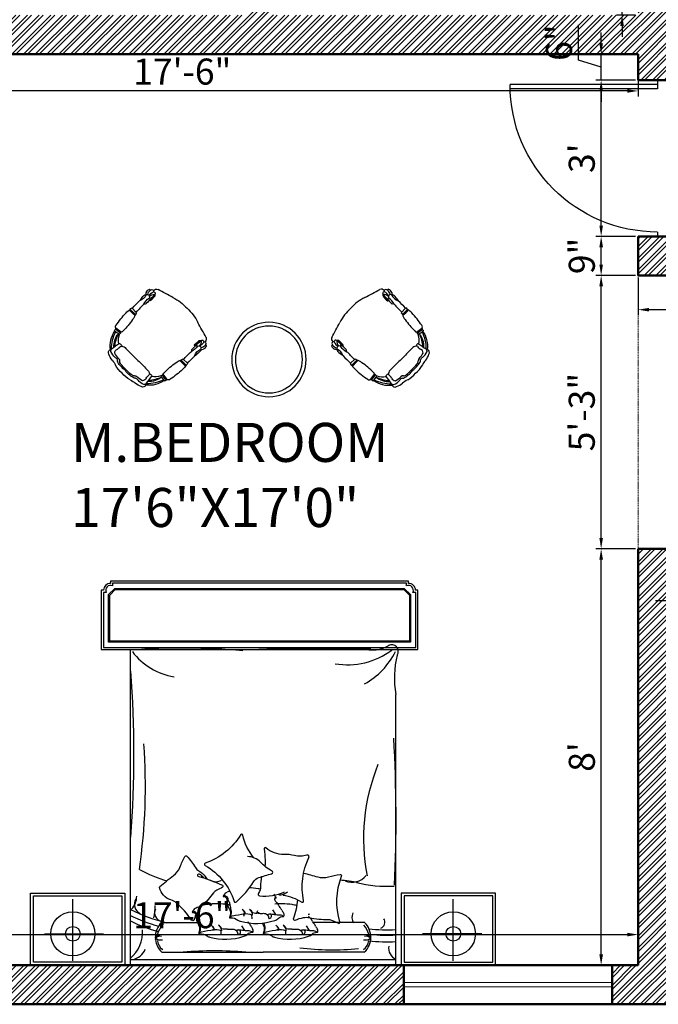
# Model space of a CAD drawing. Units: inches. Extents: x 3590 to 5167, y 65 to 1917.
# Tile 8 of 100: x 4497 to 4644, y 109 to 336. Entities that reach past the tile are written whole.
import ezdxf

# ---------------------------------------------------------------- set-up
doc = ezdxf.new("R2010")
doc.units = ezdxf.units.IN
doc.linetypes.add('DASHED', pattern=[0.75, 0.5, -0.25])
for name, color, linetype, lineweight in [('A-ANNO-DIMS', 2, 'Continuous', 18), ('A-AREA-IDEN', 7, 'Continuous', 18), ('A-DOOR', 3, 'Continuous', 25), ('A-FURN', 21, 'Continuous', 18), ('A-GLAZ', 4, 'Continuous', 18), ('A-WALL', 7, 'Continuous', 50), ('A-WALL-PATT', 251, 'Continuous', 13), ('S-BEAM-OVHD', 7, 'DASHED', 18)]:
    doc.layers.add(name, color=color, linetype=linetype, lineweight=lineweight)
for name, color, linetype in [('FUR', 42, 'Continuous'), ('furn', 7, 'Continuous'), ('HA-FUR', 8, 'Continuous'), ('HA-P', 8, 'Continuous'), ('SAN', 5, 'Continuous'), ('wood', 26, 'Continuous')]:
    doc.layers.add(name, color=color, linetype=linetype)
doc.styles.get("Standard").update_dxf_attribs({"font": 'arial.ttf'})
doc.dimstyles.new('ISO-25', dxfattribs={"dimtxt": 9, "dimasz": 2.5, "dimexe": 1.25, "dimexo": 0.625, "dimtad": 1, "dimdec": 1, "dimlunit": 3, "dimtxsty": 'Standard', "dimcen": 2.5, "dimadec": 0, "dimazin": 0, "dimtfac": 1, "dimtdec": 1, "dimtmove": 0, "dimatfit": 3, "dimfxl": 1, "dimarcsym": 0})

# ---------------------------------------------------------------- blocks, each defined once
blk = doc.blocks.new('D1')
for p, q in [((1, 0), (1, 34)), ((2, 0), (2, 33.99)), ((0, 0), (2, 0)), ((35, 0), (36, 0))]:
    blk.add_line(p, q)
at = {"ltscale": 0.5}
blk.add_arc((1, 0), 34, 0, 90, dxfattribs=at)
blk = doc.blocks.new('*D262')
at = {"layer": 'A-ANNO-DIMS', "color": 0, "lineweight": -2, "transparency": 16777216}
for p, q in [((4635.58, 345.56), (4635.58, 356.24)), ((4638.65, 343.06), (4634.33, 343.06)), ((4635.58, 337.06), (4635.58, 343.06)), ((4638.65, 337.06), (4634.33, 337.06)), ((4635.58, 334.56), (4635.58, 332.06))]:
    blk.add_line(p, q, dxfattribs=at)
at = {"layer": 'A-ANNO-DIMS', "color": 0, "transparency": 16777216}
for points in [[(4635.17, 345.56), (4636, 345.56), (4635.58, 343.06)], [(4635.17, 334.56), (4636, 334.56), (4635.58, 337.06)]]:
    blk.add_solid(points, dxfattribs=at)
at = {"layer": 'Defpoints', "color": 0, "transparency": 16777216}
for p in [(4635.58, 343.06), (4639.27, 343.06), (4639.27, 337.06)]:
    blk.add_point(p, dxfattribs=at)
at = {"layer": 'A-ANNO-DIMS', "color": 0, "transparency": 16777216, "insert": (4631.89, 352.15), "char_height": 6, "attachment_point": 5, "rotation": 90}
blk.add_mtext('6"', dxfattribs=at)
blk = doc.blocks.new('*D265')
at = {"layer": 'A-ANNO-DIMS', "color": 0, "lineweight": -2, "transparency": 16777216}
for p, q in [((4429.27, 327.43), (4429.27, 318.33)), ((4639.27, 327.43), (4639.27, 318.33)), ((4636.77, 319.58), (4431.77, 319.58))]:
    blk.add_line(p, q, dxfattribs=at)
at = {"layer": 'A-ANNO-DIMS', "color": 0, "transparency": 16777216}
for points in [[(4431.77, 319.99), (4431.77, 319.16), (4429.27, 319.58)], [(4636.77, 319.99), (4636.77, 319.16), (4639.27, 319.58)]]:
    blk.add_solid(points, dxfattribs=at)
at = {"layer": 'Defpoints', "color": 0, "transparency": 16777216}
for p in [(4429.27, 328.06), (4639.27, 328.06), (4429.27, 319.58)]:
    blk.add_point(p, dxfattribs=at)
at = {"layer": 'A-ANNO-DIMS', "color": 0, "transparency": 16777216, "insert": (4534.27, 323.26), "char_height": 6, "attachment_point": 5}
blk.add_mtext('17\'-6"', dxfattribs=at)
blk = doc.blocks.new('*D225')
at = {"layer": 'A-ANNO-DIMS', "color": 0, "lineweight": -2, "transparency": 16777216}
for p, q in [((4429.27, 118.68), (4429.27, 126.38)), ((4431.77, 125.13), (4636.77, 125.13)), ((4639.27, 118.68), (4639.27, 126.38))]:
    blk.add_line(p, q, dxfattribs=at)
at = {"layer": 'A-ANNO-DIMS', "color": 0, "transparency": 16777216}
for points in [[(4431.77, 125.55), (4431.77, 124.71), (4429.27, 125.13)], [(4636.77, 125.55), (4636.77, 124.71), (4639.27, 125.13)]]:
    blk.add_solid(points, dxfattribs=at)
at = {"layer": 'Defpoints', "color": 0, "transparency": 16777216}
for p in [(4639.27, 125.13), (4429.27, 118.06), (4639.27, 118.06)]:
    blk.add_point(p, dxfattribs=at)
at = {"layer": 'A-ANNO-DIMS', "color": 0, "transparency": 16777216, "insert": (4534.27, 128.82), "char_height": 6, "attachment_point": 5}
blk.add_mtext('17\'-6"', dxfattribs=at)
blk = doc.blocks.new('*D226')
at = {"layer": 'A-ANNO-DIMS', "color": 0, "lineweight": -2, "transparency": 16777216}
for p, q in [((4638.65, 214.06), (4629.51, 214.06)), ((4630.76, 120.56), (4630.76, 211.56)), ((4638.65, 118.06), (4629.51, 118.06))]:
    blk.add_line(p, q, dxfattribs=at)
at = {"layer": 'A-ANNO-DIMS', "color": 0, "transparency": 16777216}
for points in [[(4630.35, 211.56), (4631.18, 211.56), (4630.76, 214.06)], [(4630.35, 120.56), (4631.18, 120.56), (4630.76, 118.06)]]:
    blk.add_solid(points, dxfattribs=at)
at = {"layer": 'Defpoints', "color": 0, "transparency": 16777216}
for p in [(4630.76, 214.06), (4639.27, 214.06), (4639.27, 118.06)]:
    blk.add_point(p, dxfattribs=at)
at = {"layer": 'A-ANNO-DIMS', "color": 0, "transparency": 16777216, "insert": (4627.08, 166.06), "char_height": 6, "attachment_point": 5, "rotation": 90}
blk.add_mtext("8'", dxfattribs=at)
blk = doc.blocks.new('*D227')
at = {"layer": 'A-ANNO-DIMS', "color": 0, "lineweight": -2, "transparency": 16777216}
for p, q in [((4638.65, 277.06), (4629.51, 277.06)), ((4630.76, 216.56), (4630.76, 274.56)), ((4638.65, 214.06), (4629.51, 214.06))]:
    blk.add_line(p, q, dxfattribs=at)
at = {"layer": 'A-ANNO-DIMS', "color": 0, "transparency": 16777216}
for points in [[(4630.35, 274.56), (4631.18, 274.56), (4630.76, 277.06)], [(4630.35, 216.56), (4631.18, 216.56), (4630.76, 214.06)]]:
    blk.add_solid(points, dxfattribs=at)
at = {"layer": 'Defpoints', "color": 0, "transparency": 16777216}
for p in [(4630.76, 277.06), (4639.27, 277.06), (4639.27, 214.06)]:
    blk.add_point(p, dxfattribs=at)
at = {"layer": 'A-ANNO-DIMS', "color": 0, "transparency": 16777216, "insert": (4627.07, 245.56), "char_height": 6, "attachment_point": 5, "rotation": 90}
blk.add_mtext('5\'-3"', dxfattribs=at)
blk = doc.blocks.new('*D228')
at = {"layer": 'A-ANNO-DIMS', "color": 0, "lineweight": -2, "transparency": 16777216}
for p, q in [((4638.65, 286.06), (4629.51, 286.06)), ((4630.76, 279.56), (4630.76, 283.56)), ((4638.65, 277.06), (4629.51, 277.06))]:
    blk.add_line(p, q, dxfattribs=at)
at = {"layer": 'A-ANNO-DIMS', "color": 0, "transparency": 16777216}
for points in [[(4630.35, 283.56), (4631.18, 283.56), (4630.76, 286.06)], [(4630.35, 279.56), (4631.18, 279.56), (4630.76, 277.06)]]:
    blk.add_solid(points, dxfattribs=at)
at = {"layer": 'Defpoints', "color": 0, "transparency": 16777216}
for p in [(4630.76, 286.06), (4639.27, 286.06), (4639.27, 277.06)]:
    blk.add_point(p, dxfattribs=at)
at = {"layer": 'A-ANNO-DIMS', "color": 0, "transparency": 16777216, "insert": (4627.08, 281.56), "char_height": 6, "attachment_point": 5, "rotation": 90}
blk.add_mtext('9"', dxfattribs=at)
blk = doc.blocks.new('*D177')
at = {"layer": 'A-ANNO-DIMS', "color": 0, "lineweight": -2, "transparency": 16777216}
for p, q in [((4638.65, 322.06), (4629.51, 322.06)), ((4630.76, 288.56), (4630.76, 319.56)), ((4638.65, 286.06), (4629.51, 286.06))]:
    blk.add_line(p, q, dxfattribs=at)
at = {"layer": 'A-ANNO-DIMS', "color": 0, "transparency": 16777216}
for points in [[(4630.35, 319.56), (4631.18, 319.56), (4630.76, 322.06)], [(4630.35, 288.56), (4631.18, 288.56), (4630.76, 286.06)]]:
    blk.add_solid(points, dxfattribs=at)
at = {"layer": 'Defpoints', "color": 0, "transparency": 16777216}
for p in [(4630.76, 322.06), (4639.27, 322.06), (4639.27, 286.06)]:
    blk.add_point(p, dxfattribs=at)
at = {"layer": 'A-ANNO-DIMS', "color": 0, "transparency": 16777216, "insert": (4627.07, 304.06), "char_height": 6, "attachment_point": 5, "rotation": 90}
blk.add_mtext("3'", dxfattribs=at)
blk = doc.blocks.new('*D178')
at = {"layer": 'A-ANNO-DIMS', "color": 0, "lineweight": -2, "transparency": 16777216}
for p, q in [((4625.51, 326.64), (4625.51, 334.81)), ((4630.76, 330.56), (4630.76, 333.06)), ((4638.65, 328.06), (4629.51, 328.06)), ((4630.76, 322.06), (4630.76, 328.06)), ((4630.76, 322.06), (4630.76, 328.06)), ((4630.76, 325.06), (4625.51, 326.64)), ((4638.65, 322.06), (4629.51, 322.06)), ((4630.76, 319.56), (4630.76, 317.06))]:
    blk.add_line(p, q, dxfattribs=at)
at = {"layer": 'A-ANNO-DIMS', "color": 0, "transparency": 16777216}
for points in [[(4630.35, 330.56), (4631.18, 330.56), (4630.76, 328.06)], [(4630.35, 319.56), (4631.18, 319.56), (4630.76, 322.06)]]:
    blk.add_solid(points, dxfattribs=at)
at = {"layer": 'Defpoints', "color": 0, "transparency": 16777216}
for p in [(4630.76, 328.06), (4639.27, 328.06), (4639.27, 322.06)]:
    blk.add_point(p, dxfattribs=at)
at = {"layer": 'A-ANNO-DIMS', "color": 0, "transparency": 16777216, "insert": (4621.82, 330.72), "char_height": 6, "attachment_point": 5, "rotation": 90}
blk.add_mtext('6"', dxfattribs=at)
blk = doc.blocks.new('*D179')
at = {"layer": 'A-ANNO-DIMS', "color": 0, "lineweight": -2, "transparency": 16777216}
for p, q in [((4639.27, 276.43), (4639.27, 267.91)), ((4687.27, 276.43), (4687.27, 267.91)), ((4684.77, 269.16), (4641.77, 269.16))]:
    blk.add_line(p, q, dxfattribs=at)
at = {"layer": 'A-ANNO-DIMS', "color": 0, "transparency": 16777216}
for points in [[(4641.77, 269.57), (4641.77, 268.74), (4639.27, 269.16)], [(4684.77, 269.57), (4684.77, 268.74), (4687.27, 269.16)]]:
    blk.add_solid(points, dxfattribs=at)
at = {"layer": 'Defpoints', "color": 0, "transparency": 16777216}
for p in [(4639.27, 277.06), (4687.27, 277.06), (4639.27, 269.16)]:
    blk.add_point(p, dxfattribs=at)
at = {"layer": 'A-ANNO-DIMS', "color": 0, "transparency": 16777216, "insert": (4663.27, 272.78), "char_height": 6, "attachment_point": 5}
blk.add_mtext("4'", dxfattribs=at)
blk = doc.blocks.new('*D257')
at = {"layer": 'A-ANNO-DIMS', "color": 0, "lineweight": -2, "transparency": 16777216}
for p, q in [((4648.27, 204.43), (4648.27, 200.83)), ((4651.27, 204.43), (4651.27, 200.83)), ((4645.77, 202.08), (4643.27, 202.08)), ((4648.27, 202.08), (4651.27, 202.08)), ((4653.77, 202.08), (4664.42, 202.08))]:
    blk.add_line(p, q, dxfattribs=at)
at = {"layer": 'A-ANNO-DIMS', "color": 0, "transparency": 16777216}
for points in [[(4645.77, 202.49), (4645.77, 201.66), (4648.27, 202.08)], [(4653.77, 202.49), (4653.77, 201.66), (4651.27, 202.08)]]:
    blk.add_solid(points, dxfattribs=at)
at = {"layer": 'Defpoints', "color": 0, "transparency": 16777216}
for p in [(4648.27, 205.06), (4651.27, 205.06), (4651.27, 202.08)]:
    blk.add_point(p, dxfattribs=at)
at = {"layer": 'A-ANNO-DIMS', "color": 0, "transparency": 16777216, "insert": (4660.35, 205.77), "char_height": 6, "attachment_point": 5}
blk.add_mtext('3"', dxfattribs=at)
blk = doc.blocks.new('A$C0A42580C')
at = {"layer": 'SAN'}
for p, q in [((0.2873, 0.0301), (0.2873, 0.4484)), ((2.8678, 0.0301), (2.8678, 0.4484)), ((0.0949, 0.2135), (0.4958, 0.2135)), ((3.0601, 0.2135), (2.6592, 0.2135))]:
    blk.add_line(p, q, dxfattribs=at)
for centre, radius in [((0.2873, 0.2135), 0.15), ((2.8678, 0.2135), 0.15), ((0.2873, 0.2135), 0.05), ((2.8678, 0.2135), 0.05)]:
    blk.add_circle(centre, radius, dxfattribs=at)
at = {"layer": 'wood'}
for p, q in [((0.6775, 0.8851), (0.6775, 2.1392)), ((2.4775, 0.8016), (2.4775, 1.838)), ((2.4775, 0), (2.4775, 0.8016)), ((1.5, 0.3423), (1.5016, 0.3142)), ((1.6633, 0.3438), (1.6434, 0.3761)), ((0.888, 0.289), (1.1327, 0.289)), ((1.4538, 0.2362), (1.434, 0.2685)), ((1.8919, 0.2362), (1.8721, 0.2685)), ((2.267, 0.289), (1.9163, 0.289)), ((1.2906, 0.2348), (1.2921, 0.2067)), ((1.7287, 0.2348), (1.7302, 0.2067)), ((0.8909, 0.089), (1.5775, 0.089)), ((2.2642, 0.089), (1.5775, 0.089)), ((0.6775, 0.039), (2.4775, 0.039)), ((0.6775, 0), (2.4775, 0))]:
    blk.add_line(p, q, dxfattribs=at)
blk.add_lwpolyline([(0.6775, 0), (0.6775, 0.8851)], dxfattribs=at)
for points in [[(1.516, 0.7294, -0.128392), (1.4401, 0.8834, 0.70791), (1.427, 0.8863, -0.16964), (1.1848, 0.6919, 0.664036), (1.184, 0.6776, -0.184649), (1.3819, 0.4332, 0.662242), (1.3969, 0.4309, 0.078539), (1.5137, 0.5669, -0.1736), (1.5484, 0.5947, -0.02159), (1.6357, 0.6205, 0.697276), (1.6379, 0.6405, -0.093019), (1.5606, 0.699, 0.216632), (1.4719, 0.7371, -2.511293)], [(1.1211, 0.3454, 0.032543), (1.1095, 0.3091, -0.658965), (1.0917, 0.3063, 0.074753), (0.9887, 0.4234, 0.100988), (0.953, 0.4429, -0.270711), (0.8753, 0.5273, -0.276825), (0.8775, 0.5337, -0.014937), (0.9701, 0.6081, 0.134834), (1.0135, 0.6643, -0.023706), (1.0474, 0.7372, -0.664036), (1.0616, 0.7394, -0.035987), (1.119, 0.6627, 0.118631), (1.1415, 0.6412, -0.132738), (1.1955, 0.5864)], [(1.6795, 0.4818, 0.263265), (1.7191, 0.4839, -0.026108), (1.743, 0.4973, 0.027613), (1.7137, 0.4764, -0.089259), (1.8403, 0.429, 0.662242), (1.8528, 0.4376, -0.162037), (1.8882, 0.732, 0.676499), (1.8733, 0.748, -0.160513), (1.7901, 0.7439, 0.07473), (1.7202, 0.7523, -0.187721), (1.5966, 0.7963, 0.70791), (1.5851, 0.7895, -0.010003), (1.5921, 0.7143, -0.07079), (1.5891, 0.6719, 0.099539)], [(1.1759, 0.5928, 0.013884), (1.1549, 0.6131, 0.174178), (1.1437, 0.6177, 0.104076), (1.1358, 0.6165, 0.389829), (1.1324, 0.6097, 0.296089), (1.1415, 0.6019, -0.036701), (1.1572, 0.5985, -0.040547), (1.3022, 0.543, -0.70791), (1.3021, 0.5296, -0.016811), (1.2631, 0.5085, 0.11866), (1.2414, 0.4904, -0.048791), (1.1649, 0.4055, 0.103757)], [(1.8113, 0.4446, -0.069098), (1.7831, 0.3187, 0.658965), (1.7961, 0.3062, -0.049789), (1.8516, 0.3234, -0.103757), (1.8905, 0.3233, 0.055725), (2.0203, 0.3103, -0.11866), (2.0478, 0.304, 0.016811), (2.0881, 0.2856, 0.70791), (2.0989, 0.2936, -0.16964), (2.1104, 0.604, 0.664036), (2.1001, 0.6139, 0.023706), (2.0214, 0.597, -0.134834), (1.9505, 0.5976, 0.012748), (1.8522, 0.6228)], [(1.5674, 0.601, 0.057807), (1.5606, 0.5339, -0.173425), (1.5457, 0.49, 0.589988), (1.5538, 0.4706, 0.137312), (1.7236, 0.4985, 0.137312)], [(1.3107, 0.4764, 0.145733), (1.3069, 0.4677, 0.488583), (1.3089, 0.4657, -0.012138), (1.3131, 0.4661, -0.125673), (1.3213, 0.4646, -0.750706)], [(1.3153, 0.4751, -0.274893), (1.3379, 0.4529, 0.051436), (1.3468, 0.4293, -0.086628), (1.3532, 0.4078, 0.040196), (1.3593, 0.3772, -0.184744), (1.3556, 0.3344, -2.554464)], [(1.317, 0.4683, -0.060098), (1.3283, 0.4571, -0.16247), (1.3313, 0.4487, 0.120018), (1.3493, 0.3815, -0.060072), (1.3541, 0.3695, -0.13107), (1.3541, 0.3395, -0.024415), (1.3534, 0.3373, 0.070398), (1.3503, 0.3233, 0.528689), (1.3524, 0.3216, -0.069388), (1.3557, 0.3222, -0.158233), (1.4075, 0.3065, 0.085461), (1.4255, 0.2981, 0.147196), (1.6571, 0.3041, 0.10985), (1.6823, 0.3191, -0.179095), (1.7126, 0.3319, -2.318897)], [(1.1013, 0.3688, 0.145733), (1.0975, 0.3601, 0.488583), (1.0995, 0.3581, -0.012138), (1.1036, 0.3585, -0.125673), (1.1119, 0.357, -0.750706)], [(1.1059, 0.3675, -0.274893), (1.1285, 0.3453, 0.051436), (1.1373, 0.3217, -0.086628), (1.1438, 0.3003, 0.040196), (1.1499, 0.2696, -0.184744), (1.1462, 0.2269, -2.554464)], [(1.1076, 0.3607, -0.060098), (1.1189, 0.3495, -0.16247), (1.1219, 0.3411, 0.120018), (1.1399, 0.2739, -0.060072), (1.1447, 0.2619, -0.13107), (1.1447, 0.2319, -0.024415), (1.144, 0.2297, 0.070398), (1.1409, 0.2157, 0.528689), (1.143, 0.2141, -0.069388), (1.1463, 0.2146, -0.158233), (1.1981, 0.1989, 0.085461), (1.2161, 0.1905, 0.147196), (1.4477, 0.1965, 0.10985), (1.4728, 0.2115, -0.179095), (1.5032, 0.2244, -2.318897)], [(1.3509, 0.3219, -0.117141), (1.3688, 0.335, -0.025084), (1.4533, 0.348, 0.033691)], [(1.4359, 0.3803, -0.198519), (1.452, 0.3494, 0.826402), (1.4558, 0.349, 0.095956), (1.4561, 0.3528, 0.242899), (1.4461, 0.3686, -17.523452)], [(1.5447, 0.3525, -0.083557), (1.507, 0.3546, 0.203162), (1.4851, 0.3792, -0.208037), (1.5043, 0.3409, 0.124669), (1.4432, 0.3469, 0.965934)], [(1.5394, 0.3688, 0.145733), (1.5356, 0.3601, 0.488583), (1.5376, 0.3581, -0.012138), (1.5418, 0.3585, -0.125673), (1.55, 0.357, -0.750706)], [(1.5447, 0.3525, -0.008229), (1.5728, 0.3519, 0.033691)], [(1.5728, 0.3519, -0.46905), (1.6152, 0.321, 0.420988), (1.62, 0.3169, 0.857652), (1.6221, 0.3484, 0.548526)], [(1.603, 0.3451, -0.099719), (1.6221, 0.3484, 0.102691)], [(1.6214, 0.3487, -0.010168), (1.6558, 0.3447, 0.033691), (1.6907, 0.3423, -0.220869), (1.7148, 0.3311, -0.288972)], [(1.2265, 0.2728, -0.198519), (1.2426, 0.2418, 0.826402), (1.2463, 0.2415, 0.095956), (1.2467, 0.2452, 0.242899), (1.2366, 0.2611, -17.523452)], [(1.3353, 0.2449, -0.083557), (1.2976, 0.247, 0.203162), (1.2757, 0.2717, -0.208037), (1.2948, 0.2333, 0.124669), (1.2338, 0.2393, 0.965934)], [(1.5721, 0.286, 0.022869), (1.578, 0.2739, -0.060072), (1.5828, 0.2619, -0.13107), (1.5828, 0.2319, -0.024415), (1.5821, 0.2297, 0.070398), (1.579, 0.2157, 0.528689), (1.5811, 0.2141, -0.069388), (1.5844, 0.2146, -0.158233), (1.6362, 0.1989, 0.085461), (1.6542, 0.1905, 0.147196), (1.8858, 0.1965, 0.10985), (1.911, 0.2115, -0.179095), (1.9413, 0.2244, -2.318897)], [(1.5838, 0.2873, 0.023398), (1.588, 0.2696, -0.184744), (1.5843, 0.2269, -2.554464)], [(1.6646, 0.2728, -0.198519), (1.6807, 0.2418, 0.826402), (1.6845, 0.2415, 0.095956), (1.6848, 0.2452, 0.242899), (1.6748, 0.2611, -17.523452)], [(1.7734, 0.2449, -0.083557), (1.7357, 0.247, 0.203162), (1.7138, 0.2717, -0.208037), (1.733, 0.2333, 0.124669), (1.6719, 0.2393, 0.965934)], [(1.1415, 0.2143, -0.117141), (1.1594, 0.2274, -0.025084), (1.2439, 0.2405, 0.033691)], [(1.3353, 0.2449, -0.008229), (1.3633, 0.2443, 0.033691)], [(1.3633, 0.2443, -0.46905), (1.4058, 0.2134, 0.420988), (1.4106, 0.2093, 0.857652), (1.4127, 0.2408, 0.548526)], [(1.3936, 0.2375, -0.099719), (1.4127, 0.2408, 0.102691)], [(1.412, 0.2411, -0.010168), (1.4464, 0.2371, 0.033691), (1.4812, 0.2348, -0.220869), (1.5054, 0.2235, -0.288972)], [(1.5796, 0.2143, -0.117141), (1.5975, 0.2274, -0.025084), (1.682, 0.2405, 0.033691)], [(1.7734, 0.2449, -0.008229), (1.8015, 0.2443, 0.033691)], [(1.8015, 0.2443, -0.46905), (1.8439, 0.2134, 0.420988), (1.8487, 0.2093, 0.857652), (1.8508, 0.2408, 0.548526)], [(1.8317, 0.2375, -0.099719), (1.8508, 0.2408, 0.102691)], [(1.8501, 0.2411, -0.010168), (1.8845, 0.2371, 0.033691), (1.9193, 0.2348, -0.220869), (1.9435, 0.2235, -0.288972)]]:
    blk.add_lwpolyline(points, format="xyb", dxfattribs=at)
for points in [[(0.64, 0), (0, 0), (0, 0.49), (0.64, 0.49)], [(0.62, 0.02), (0.02, 0.02), (0.02, 0.47), (0.62, 0.47)], [(2.515, 0), (3.155, 0), (3.155, 0.49), (2.515, 0.49)], [(2.535, 0.02), (3.135, 0.02), (3.135, 0.47), (2.535, 0.47)]]:
    blk.add_lwpolyline(points, close=True, dxfattribs=at)
for centre, radius, start, end in [((1.0344, -2.14), 4.292, 84.56078, 94.7164), ((2.0208, -11.0786), 13.2288, 88.75549, 92.51133), ((2.1491, 2.5471), 0.5083, 260.65485, 306.44155), ((2.3125, 2.3833), 0.2443, 254.1515, 300.95574), ((2.4501, 2.1309), 0.0445, 324.18954, 118.92203), ((1.0494, 2.4026), 0.4515, 217.47941, 260.35986), ((2.0168, 2.3573), 0.5127, 299.08175, 333.44367), ((3.1371, 1.9502), 0.669, 166.6404, 189.65708), ((-7.0839, 1.4328), 7.7858, 355.84817, 4.15183), ((-7.2439, 0.9937), 9.7233, 357.34474, 3.23068), ((-3.167, 1.2143), 3.9465, 351.77286, 4.18386), ((3.5803, 0.8622), 1.3213, 157.81295, 191.15154), ((1.1611, 1.4181), 0.8768, 241.21362, 254.41879), ((2.181, 0.6859), 0.1221, 247.37754, 321.13165), ((1.2583, 0.6364), 0.0695, 238.58923, 301.92671), ((1.7861, -2.1601), 2.7557, 80.89877, 83.46656), ((2.4192, 1.3819), 0.8461, 255.77539, 273.25587), ((0.5904, 0.4689), 0.13, 317.38218, 359.70393), ((1.3546, 0.4469), 0.0529, 114.21284, 146.15395), ((2.6126, -2.3504), 3.1201, 113.83178, 114.21284), ((1.4714, 0.0722), 0.4528, 80.62397, 88.74059), ((1.4035, -0.3388), 0.8693, 79.71489, 80.62397), ((1.6301, 0.4539), 0.0342, 31.14095, 54.95422), ((1.5664, 0.4154), 0.1086, 24.20989, 31.14095), ((0.7723, 0.4131), 0.0674, 147.68233, 245.79865), ((0.0312, 0.4583), 0.8174, 350.42368, 356.2506), ((2.4032, -2.458), 3.1201, 113.55686, 114.21284), ((1.2046, 0.2912), 0.121, 99.42032, 113.55686), ((1.2774, -0.1478), 0.5659, 95.90379, 99.42032), ((1.2626, -0.005), 0.4223, 88.74059, 95.90379), ((1.2619, -0.0354), 0.4528, 80.62397, 88.74059), ((1.1941, -0.4464), 0.8693, 79.45871, 80.62397), ((1.6709, 0.4489), 0.0156, 131.9623, 212.08127), ((1.6729, 0.4422), 0.0178, 140.41793, 157.63267), ((1.7007, -0.005), 0.4223, 88.74059, 95.90379), ((1.7235, 0.4818), 0.0777, 212.08127, 227.364), ((1.6635, 0.4499), 0.00568, 95.52245, 140.41793), ((1.6627, 0.4587), 0.00309, 275.52245, 24.20989), ((1.6391, 0.3902), 0.0469, 17.32618, 47.364), ((1.7106, 0.4125), 0.028, 197.32618, 226.17302), ((1.7001, -0.0354), 0.4528, 80.62397, 88.74059), ((1.6322, -0.4464), 0.8693, 78.43923, 80.62397), ((1.1611, 1.3191), 1.0568, 242.76671, 257.10398), ((1.1611, 1.3191), 1.0937, 243.75553, 254.4906), ((0.9021, 0.3562), 0.0605, 155.8342, 254.41058), ((1.1452, 0.3394), 0.0529, 114.21284, 146.15395), ((1.4207, 0.3463), 0.0342, 31.14095, 54.95422), ((1.4614, 0.3413), 0.0156, 131.9623, 212.08127), ((1.4635, 0.3347), 0.0178, 140.41793, 157.63267), ((1.4541, 0.3424), 0.00568, 95.52245, 140.41793), ((1.357, 0.3078), 0.1086, 24.20989, 31.14095), ((1.4533, 0.3511), 0.00309, 275.52245, 24.20989), ((1.6431, 0.3422), 0.0695, 26.61764, 46.17302), ((1.8202, 0.431), 0.1287, 206.61764, 215.96192), ((1.6975, 0.3419), 0.023, 350.76434, 35.96192), ((1.7058, 0.3406), 0.0145, 328.02977, 350.76434), ((1.9016, 0.3347), 0.0178, 140.41793, 157.63267), ((1.8922, 0.3424), 0.00568, 95.52245, 140.41793), ((2.2511, 0.3256), 0.071, 155.86842, 211.04513), ((1.1611, 1.2816), 1.0937, 243.75553, 254.38927), ((0.9846, 0.1903), 0.1381, 134.39284, 227.23745), ((0.9986, 0.1735), 0.1427, 136.58239, 164.9725), ((1.5012, 0.305), 0.028, 197.32618, 226.17302), ((1.4337, 0.2347), 0.0695, 26.61764, 46.17302), ((1.715, 0.3349), 0.00379, 207.1817, 328.02977), ((1.9522, 0.3743), 0.0777, 212.08127, 227.364), ((1.8678, 0.2827), 0.0469, 17.32618, 47.364), ((1.9393, 0.305), 0.028, 197.32618, 226.17302), ((1.8718, 0.2347), 0.0695, 26.61764, 46.17302), ((2.1565, 0.1735), 0.1427, 15.0275, 43.41761), ((2.1704, 0.1903), 0.1381, 312.76255, 45.60716), ((2.3616, 0.2915), 0.0419, 290.78583, 35.36309), ((0.5293, 0.2241), 0.2307, 309.63048, 4.27465), ((0.8698, 0.1793), 0.0229, 77.14902, 159.1786), ((1.6108, 0.3235), 0.1287, 206.61764, 215.96192), ((1.5055, 0.2273), 0.00379, 207.1817, 328.02977), ((1.4881, 0.2344), 0.023, 350.76434, 35.96192), ((1.4964, 0.233), 0.0145, 328.02977, 350.76434), ((2.0489, 0.3235), 0.1287, 206.61764, 215.96192), ((1.9436, 0.2273), 0.00379, 207.1817, 328.02977), ((1.9262, 0.2344), 0.023, 350.76434, 35.96192), ((1.9345, 0.233), 0.0145, 328.02977, 350.76434), ((2.2853, 0.1793), 0.0229, 20.8214, 102.85098), ((2.4192, 1.2667), 1.0261, 263.09035, 273.25587), ((2.4192, 1.2667), 1.0629, 263.94374, 273.25587), ((0.8396, 0.185), 0.0112, 314.89662, 45.10338), ((0.8413, 0.1846), 0.0128, 299.47062, 57.44416), ((0.8844, 0.2286), 0.0569, 229.70587, 281.11527), ((0.8802, 0.1371), 0.0592, 81.47786, 123.11925), ((0.9466, 0.1765), 0.0862, 185.53723, 234.68694), ((2.2085, 0.1765), 0.0862, 305.31306, 354.46277), ((2.2706, 0.2286), 0.0569, 258.88473, 310.29413), ((2.2749, 0.1371), 0.0592, 56.88075, 98.52214), ((2.4192, 1.2218), 1.0629, 263.23622, 273.25587), ((2.3138, 0.1846), 0.0128, 122.55584, 240.52938), ((2.3154, 0.185), 0.0112, 134.89662, 225.10338), ((0.6729, 0.151), 0.1135, 279.23824, 338.73819), ((1.2481, -2.5919), 2.6893, 85.4722, 94.5278), ((2.0447, 1.7022), 1.5979, 262.13639, 276.48786), ((2.508, 0.1152), 0.0792, 169.94668, 248.24015)]:
    blk.add_arc(centre, radius, start, end, dxfattribs=at)
blk = doc.blocks.new('A$C623F1DA0')
at = {"layer": 'FUR'}
blk.add_lwpolyline([(0.628, 2.912, 0.414214), (0.562, 2.978), (0.562, 3), (0, 3), (0, 0), (0.562, 0), (0.562, 0.022, 0.414214), (0.628, 0.088), (0.65, 0.088), (0.65, 2.912)], format="xyb", close=True, dxfattribs=at)
at = {"layer": 'HA-FUR'}
blk.add_lwpolyline([(0.6034, 2.892, 0.710288), (0.542, 2.9534), (0.542, 2.98), (0.02, 2.98), (0.02, 0.02), (0.542, 0.02), (0.542, 0.0466, 0.710288), (0.6034, 0.108), (0.63, 0.108), (0.63, 2.892)], format="xyb", close=True, dxfattribs=at)
at = {"layer": 'HA-P'}
for points in [[(0.07, 2.93), (0.5213, 2.93), (0.58, 2.8713), (0.58, 0.1287), (0.5213, 0.07), (0.07, 0.07)], [(0.08, 2.92), (0.5171, 2.92), (0.57, 2.8671), (0.57, 0.1329), (0.5171, 0.08), (0.08, 0.08)]]:
    blk.add_lwpolyline(points, close=True, dxfattribs=at)
blk = doc.blocks.new('CHAIR6')
at = {"layer": 'furn'}
for p, q in [((0.41, 0.26), (0.4094, 0.3185)), ((0.4281, 0.3181), (0.4272, 0.263)), ((0.41, -0.26), (0.4094, -0.3185)), ((0.4281, -0.3181), (0.4272, -0.263))]:
    blk.add_line(p, q, dxfattribs=at)
for centre in [(0.4053, 0.3148), (0.2174, 0.2867), (0.2187, 0.2766), (0.22, 0.2683), (0.2209, 0.2599), (0.2221, 0.2517), (0.2231, 0.2433), (0.4052, 0.3065), (0.4053, 0.2897), (0.4054, 0.2981), (0.4054, 0.2729), (0.4055, 0.2812), (0.4056, 0.2643), (0.2174, -0.2867), (0.2187, -0.2766), (0.22, -0.2683), (0.2209, -0.2599), (0.2221, -0.2517), (0.2231, -0.2433), (0.4052, -0.3065), (0.4053, -0.2897), (0.4053, -0.3148), (0.4054, -0.2981), (0.4054, -0.2729), (0.4055, -0.2812), (0.4056, -0.2643)]:
    blk.add_circle(centre, 0.00425, dxfattribs=at)
for centre, radius, start, end in [((0.3719, -0.3167), 0.6382, 90.6066, 102.05541), ((0.3772, 0.1685), 0.1534, 77.89638, 94.52684), ((3.3638, 0.3149), 2.9628, 179.90105, 181.14792), ((0.4178, 0.2794), 0.04, 75.21702, 102.18253), ((0.5573, 0.1986), 0.1211, 80.56871, 102.58021), ((0.569, 0.3057), 0.0148, 11.93121, 56.71364), ((0.5574, 0.3682), 0.0592, 293.70731, 312.31146), ((0.6147, 0.2731), 0.0542, 72.72663, 108.72189), ((0.6287, 0.3179), 0.00734, 318.72654, 73.20464), ((0.2315, 0.0781), 0.2058, 99.53594, 142.96968), ((0.288, -0.009), 0.2959, 107.467, 135.69066), ((0.2204, 0.0839), 0.1637, 95.98601, 137.80844), ((0.2974, -0.0268), 0.2892, 108.96584, 130.74832), ((0.1998, 0.3299), 0.0425, 267.37882, 299.53851), ((0.5076, 0.3087), 0.3105, 183.92135, 193.66405), ((0.217, 0.2087), 0.0298, 85.88245, 112.38941), ((0.91, 0.35), 0.6998, 184.95819, 189.17441), ((0.2036, 0.356), 0.1186, 277.54736, 281.93488), ((0.2369, 0.2913), 0.0162, 83.97727, 174.0092), ((2.2364, 0.5463), 2.0315, 187.16408, 188.67417), ((0.2433, 0.2647), 0.029, 238.53775, 274.93529), ((0.2506, 0.8795), 0.6438, 269.57373, 280.24813), ((0.357, 0.3514), 0.1057, 274.42127, 300.14813), ((0.4118, 0.3013), 0.0413, 267.60688, 291.9537), ((0.4709, 1.0442), 0.7753, 266.77935, 273.30843), ((0.4807, -0.3094), 0.6241, 87.1388, 94.84242), ((0.5163, 0.348), 0.0344, 262.5365, 295.12391), ((0.5543, 0.4048), 0.1004, 244.96152, 286.92621), ((0.5583, 0.1491), 0.1284, 78.32163, 109.43704), ((0.5171, 0.2599), 0.0105, 7.92951, 98.404), ((0.5475, 0.4175), 0.1574, 262.69111, 279.4279), ((0.5763, 0.2592), 0.00554, 151.0446, 320.63906), ((0.5726, 0.2536), 0.00119, 58.88827, 217.83169), ((0.5864, 0.2986), 0.0481, 252.15364, 277.04405), ((0.5749, 0.272), 0.00992, 261.06044, 17.03518), ((0.6, 0.6108), 0.3491, 266.32513, 275.76594), ((0.5857, 0.2587), 0.00592, 143.235, 315.8485), ((0.5811, 0.2921), 0.0168, 1.95853, 81.75781), ((0.5706, 0.2994), 0.0282, 299.26311, 346.05528), ((0.54, 0.2614), 0.0504, 352.19447, 0.49312), ((0.5958, 0.265), 0.012, 240.91565, 292.3604), ((0.5993, 0.2232), 0.0286, 84.23587, 104.22566), ((0.6205, 0.2416), 0.0492, 62.08685, 124.06689), ((0.5958, 0.2324), 0.05, 38.36456, 93.27362), ((0.6272, 0.2528), 0.0606, 83.33143, 123.59051), ((0.6298, 0.2592), 0.03, 175.25421, 190.14236), ((0.6039, 0.2608), 0.00773, 242.68072, 299.22641), ((0.6055, 0.322), 0.0704, 267.27867, 279.33441), ((0.6233, 0.2599), 0.0167, 173.50236, 200.39748), ((0.6103, 0.2582), 0.0049, 236.84733, 330.71615), ((0.6462, 0.2619), 0.0322, 179.91617, 191.03659), ((0.6177, 0.2574), 0.00347, 207.27606, 12.12043), ((0.6201, 0.2638), 0.0117, 254.38571, 324.07897), ((0.7103, 0.267), 0.0896, 182.99093, 185.70819), ((0.6264, 0.2651), 0.00881, 232.86154, 349.28828), ((0.6327, 0.2954), 0.0177, 352.68742, 85.29917), ((0.6348, 0.276), 0.0126, 270.96281, 46.15927), ((0.6241, 0.3083), 0.0303, 309.85115, 329.87174), ((0.651, 0.2582), 0.0349, 27.02079, 91.1191), ((5.5909, 1.6415), 5.0957, 195.56602, 197.11239), ((0.1754, 0.1139), 0.1594, 153.58586, 173.67646), ((0.0568, 0.1796), 0.0247, 65.10842, 167.8729), ((0.2078, 0.1391), 0.1575, 161.79448, 183.48135), ((0.076, 0.1763), 0.0215, 90.49656, 146.04111), ((0.0747, 0.2065), 0.00875, 210.7256, 277.12246), ((0.0962, 0.1341), 0.0336, 65.79003, 135.37187), ((1.2944, 7.3493), 7.2545, 260.32992, 260.96162), ((0.1315, 0.2333), 0.0718, 252.51235, 277.4747), ((0.1416, 0.1481), 0.0139, 39.59763, 92.78598), ((0.2701, 0.1022), 0.1479, 115.74239, 145.5422), ((0.1013, 0.1754), 0.0542, 340.13538, 9.97368), ((0.2403, 0.0222), 0.2414, 165.22851, 185.28449), ((-0.0992, 0.1308), 0.1161, 336.07618, 0.28835), ((0.2703, 0.0325), 0.2394, 166.65717, 187.80685), ((0.064, 0.0801), 0.0277, 124.74206, 163.83274), ((0.0904, 0.0544), 0.0465, 139.20017, 173.50108), ((0.0085, 0.1198), 0.0432, 336.84052, 13.12552), ((0.0425, 0.1014), 0.0209, 307.26707, 6.28043), ((0.2344, 0.1031), 0.1711, 161.37859, 179.7853), ((0.1123, 0.1263), 0.0505, 352.81567, 37.47081), ((-4.0332, 0.095), 4.1956, 358.70239, 0.34145), ((0.3444, 0.019), 0.396, 357.24911, 18.10814), ((0.4579, 0.0143), 0.4162, 173.74932, 181.97518), ((0.2403, -0.0222), 0.2414, 174.71551, 194.77149), ((0.2703, -0.0325), 0.2394, 172.19315, 193.34283), ((0.4579, -0.0143), 0.4162, 178.02482, 186.25068), ((0.0904, -0.0544), 0.0465, 186.49892, 220.79983), ((-4.0332, -0.095), 4.1956, 359.65855, 1.29761), ((0.3444, -0.019), 0.396, 341.89186, 2.75089), ((-0.0992, -0.1308), 0.1161, 359.71165, 23.92382), ((0.1754, -0.1139), 0.1594, 186.32354, 206.41414), ((0.064, -0.0801), 0.0277, 196.16726, 235.25794), ((0.0085, -0.1198), 0.0432, 346.87448, 23.15948), ((0.2078, -0.1391), 0.1575, 176.51865, 198.20552), ((0.0425, -0.1014), 0.0209, 353.71957, 52.73293), ((0.2344, -0.1031), 0.1711, 180.2147, 198.62141), ((0.0962, -0.1341), 0.0336, 224.62813, 294.20997), ((0.1416, -0.1481), 0.0139, 267.21402, 320.40237), ((0.1123, -0.1263), 0.0505, 322.52919, 7.18433), ((0.1013, -0.1754), 0.0542, 350.02632, 19.86462), ((5.5909, -1.6415), 5.0957, 162.88761, 164.43398), ((0.0568, -0.1796), 0.0247, 192.1271, 294.89158), ((0.076, -0.1763), 0.0215, 213.95889, 269.50344), ((0.0747, -0.2065), 0.00875, 82.87754, 149.2744), ((0.2315, -0.0781), 0.2058, 217.03032, 260.46406), ((1.2944, -7.3493), 7.2545, 99.03838, 99.67008), ((0.288, 0.009), 0.2959, 224.30934, 252.533), ((0.2204, -0.0839), 0.1637, 222.19156, 264.01399), ((0.2974, 0.0268), 0.2892, 229.25168, 251.03416), ((0.1315, -0.2333), 0.0718, 82.5253, 107.48765), ((0.2701, -0.1022), 0.1479, 214.4578, 244.25761), ((0.5076, -0.3087), 0.3105, 166.33595, 176.07865), ((0.217, -0.2087), 0.0298, 247.61059, 274.11755), ((0.2433, -0.2647), 0.029, 85.06471, 121.46225), ((0.2506, -0.8795), 0.6438, 79.75187, 90.42627), ((0.1998, -0.3299), 0.0425, 60.46149, 92.62118), ((0.91, -0.35), 0.6998, 170.82559, 175.04181), ((0.2036, -0.356), 0.1186, 78.06512, 82.45264), ((2.2364, -0.5463), 2.0315, 171.32583, 172.83592), ((0.2369, -0.2913), 0.0162, 185.9908, 276.02273), ((0.3719, 0.3167), 0.6382, 257.94459, 269.3934), ((0.357, -0.3514), 0.1057, 59.85187, 85.57873), ((3.3638, -0.3149), 2.9628, 178.85208, 180.09895), ((0.4118, -0.3013), 0.0413, 68.0463, 92.39312), ((0.4709, -1.0442), 0.7753, 86.69157, 93.22065), ((0.4807, 0.3094), 0.6241, 265.15758, 272.8612), ((0.5543, -0.4048), 0.1004, 73.07379, 115.03848), ((0.5163, -0.348), 0.0344, 64.87609, 97.4635), ((0.5171, -0.2599), 0.0105, 261.596, 352.07049), ((0.5583, -0.1491), 0.1284, 250.56296, 281.67837), ((0.5475, -0.4175), 0.1574, 80.5721, 97.30889), ((0.5573, -0.1986), 0.1211, 257.41979, 279.43129), ((0.5763, -0.2592), 0.00554, 39.36094, 208.9554), ((0.5726, -0.2536), 0.00119, 142.16831, 301.11173), ((0.5864, -0.2986), 0.0481, 82.95595, 107.84636), ((0.5749, -0.272), 0.00992, 342.96482, 98.93956), ((0.569, -0.3057), 0.0148, 303.28636, 348.06879), ((0.6, -0.6108), 0.3491, 84.23406, 93.67487), ((0.5857, -0.2587), 0.00592, 44.1515, 216.765), ((0.5574, -0.3682), 0.0592, 47.68854, 66.29269), ((0.5811, -0.2921), 0.0168, 278.24219, 358.04147), ((0.5706, -0.2994), 0.0282, 13.94472, 60.73689), ((0.5958, -0.265), 0.012, 67.6396, 119.08435), ((0.54, -0.2614), 0.0504, 359.50688, 7.80553), ((0.5993, -0.2232), 0.0286, 255.77434, 275.76413), ((0.5958, -0.2324), 0.05, 266.72638, 321.63544), ((0.6205, -0.2416), 0.0492, 235.93311, 297.91315), ((0.6272, -0.2528), 0.0606, 236.40949, 276.66857), ((0.6298, -0.2592), 0.03, 169.85764, 184.74579), ((0.6039, -0.2608), 0.00773, 60.77359, 117.31928), ((0.6055, -0.322), 0.0704, 80.66559, 92.72133), ((0.6233, -0.2599), 0.0167, 159.60252, 186.49764), ((0.6103, -0.2582), 0.0049, 29.28385, 123.15267), ((0.6462, -0.2619), 0.0322, 168.96341, 180.08383), ((0.6177, -0.2574), 0.00347, 347.87957, 152.72394), ((0.6201, -0.2638), 0.0117, 35.92103, 105.61429), ((0.7103, -0.267), 0.0896, 174.29181, 177.00907), ((0.6264, -0.2651), 0.00881, 10.71172, 127.13846), ((0.6287, -0.3179), 0.00734, 286.79536, 41.27346), ((0.6327, -0.2954), 0.0177, 274.70083, 7.31258), ((0.6348, -0.276), 0.0126, 313.84073, 89.03719), ((0.6241, -0.3083), 0.0303, 30.12826, 50.14885), ((0.651, -0.2582), 0.0349, 268.8809, 332.97921), ((0.3772, -0.1685), 0.1534, 265.47316, 282.10362), ((0.4178, -0.2794), 0.04, 257.81747, 284.78298), ((0.6147, -0.2731), 0.0542, 251.27811, 287.27337)]:
    blk.add_arc(centre, radius, start, end, dxfattribs=at)
blk = doc.blocks.new('A$C78847651')
at = {"layer": 'furn'}
for radius in [0.3, 0.27]:
    blk.add_circle((1.2923, 0.5659), radius, dxfattribs=at)
at = {"layer": 'furn', "rotation": 315}
blk.add_blockref('CHAIR6', (0.1103, 0.6765), dxfattribs=at)
at = {"layer": 'furn', "xscale": -1, "rotation": 44.99999999999991}
blk.add_blockref('CHAIR6', (2.4743, 0.6765), dxfattribs=at)

msp = doc.modelspace()

# ---------------------------------------------------------------- hatches: boundary and pattern name
at = {"layer": 'A-WALL-PATT', "transparency": 33554687}
h = msp.add_hatch(dxfattribs=at)
h.set_pattern_fill('ANSI32', color=256, scale=0.2)
h.set_pattern_definition([(45, (0, -1216.9392), (-1.3470384, 1.3470384), []), (45, (0.898, -1216.9392), (-1.3470384, 1.3470384), [])])
h.paths.add_polyline_path([(4684.27, 589.06), (4591.27, 589.06), (4591.27, 580.06), (4639.27, 580.06), (4639.27, 574.06), (4648.27, 574.06), (4648.27, 580.06), (4684.27, 580.06)])
h.paths.add_polyline_path([(4543.27, 589.06), (4420.27, 589.06), (4420.27, 568.06), (4429.27, 568.06), (4429.27, 580.06), (4445.92, 580.06), (4543.27, 580.06)])
h.paths.add_polyline_path([(4828.27, 589.06), (4744.27, 589.06), (4744.27, 580.06), (4828.27, 580.06)])
h.paths.add_polyline_path([(4648.27, 538.06), (4639.27, 538.06), (4639.27, 439.06), (4546.27, 439.06), (4546.27, 433.06), (4549.27, 433.06), (4549.27, 337.06), (4429.27, 337.06), (4429.27, 367.06), (4420.27, 367.06), (4420.27, 322.06), (4429.27, 322.06), (4429.27, 328.06), (4639.27, 328.06), (4639.27, 322.06), (4648.27, 322.06), (4648.27, 343.06), (4639.27, 343.06), (4639.27, 337.06), (4555.27, 337.06), (4555.27, 433.06), (4639.27, 433.06), (4639.27, 373.06), (4648.27, 373.06)])
h.paths.add_polyline_path([(4516.27, 439.06), (4429.27, 439.06), (4429.27, 520.06), (4420.27, 520.06), (4420.27, 403.06), (4429.27, 403.06), (4429.27, 433.06), (4516.27, 433.06)], flags=17)
h.paths.add_polyline_path([(5080.27, 589.06), (4888.27, 589.06), (4888.27, 580.06), (4924.27, 580.06), (4924.27, 538.06), (4933.27, 538.06), (4933.27, 580.06), (5071.27, 580.06), (5071.27, 118.06), (4933.27, 118.06), (4933.27, 349.06), (4924.27, 349.06), (4924.27, 118.06), (4898.77, 118.06), (4898.77, 109.06), (5080.27, 109.06)])
h.paths.add_polyline_path([(4933.27, 502.06), (4924.27, 502.06), (4924.27, 421.06), (4933.27, 421.06)], flags=17)
h.paths.add_polyline_path([(4802.77, 118.06), (4777.27, 118.06), (4777.27, 286.06), (4756.27, 286.06), (4756.27, 277.06), (4768.27, 277.06), (4768.27, 214.06), (4696.27, 214.06), (4696.27, 277.06), (4708.27, 277.06), (4708.27, 286.06), (4639.27, 286.06), (4639.27, 277.06), (4687.27, 277.06), (4687.27, 214.06), (4681.27, 214.06), (4681.27, 205.06), (4768.27, 205.06), (4768.27, 118.06), (4726.27, 118.06), (4726.27, 109.06), (4802.77, 109.06)])
h.paths.add_polyline_path([(4690.27, 118.06), (4648.27, 118.06), (4648.27, 135.93), (4648.27, 205.06), (4651.27, 205.06), (4651.27, 214.06), (4639.27, 214.06), (4639.27, 118.06), (4633.27, 118.06), (4633.27, 109.06), (4690.27, 109.06)])
h.paths.add_polyline_path([(4585.27, 118.06), (4584.72, 118.06), (4429.27, 118.06), (4429.27, 274.06), (4420.27, 274.06), (4420.27, 109.06), (4585.27, 109.06)])

# ---------------------------------------------------------------- linework, layer by layer
at = {"layer": 'A-GLAZ'}
for p, q in [((4633.27, 114.06), (4585.27, 114.06)), ((4633.27, 113.06), (4585.27, 113.06))]:
    msp.add_line(p, q, dxfattribs=at)
at = {"layer": 'A-WALL'}
for p, q in [((4639.27, 328.06), (4429.27, 328.06)), ((4639.27, 322.06), (4639.27, 328.06)), ((4648.27, 322.06), (4639.27, 322.06)), ((4708.27, 286.06), (4639.27, 286.06)), ((4639.27, 277.06), (4639.27, 286.06)), ((4687.27, 277.06), (4639.27, 277.06)), ((4651.27, 214.06), (4639.27, 214.06)), ((4639.27, 118.06), (4639.27, 214.06)), ((4639.27, 118.06), (4429.27, 118.06)), ((4585.27, 109.06), (4585.27, 118.06)), ((4633.27, 109.06), (4633.27, 118.06))]:
    msp.add_line(p, q, dxfattribs=at)
msp.add_lwpolyline([(5080.27, 589.06), (5080.27, 109.06), (4420.27, 109.06), (4420.27, 589.06)], close=True, dxfattribs=at)
at = {"layer": 'S-BEAM-OVHD', "ltscale": 0.5}
msp.add_line((4639.27, 277.06), (4639.27, 214.06), dxfattribs=at)

# ---------------------------------------------------------------- block references
at = {"layer": 'A-DOOR', "xscale": -1, "rotation": 90}
msp.add_blockref('D1', (4643.77, 322.06), dxfattribs=at)
at = {"layer": 'A-FURN'}
for name, p, xscale, yscale, zscale, rotation in [('A$C78847651', (4517.27, 273.86), -28.59533479380236, 28.59533479380236, 28.59533479380236, 180), ('A$C623F1DA0', (4588.53, 190.82), 24.31060204424285, 24.31060204424285, 24.31060204424285, 90)]:
    msp.add_blockref(name, p, dxfattribs=dict(at, xscale=xscale, yscale=yscale, zscale=zscale, rotation=rotation))
at = {"layer": 'A-FURN', "xscale": 33.96864568351422, "yscale": 33.96864568351422, "zscale": 33.96864568351422}
msp.add_blockref('A$C0A42580C', (4499.29, 118.06), dxfattribs=at)

# ---------------------------------------------------------------- texts
at = {"layer": 'A-AREA-IDEN', "insert": (4508.65, 243.07), "char_height": 9, "attachment_point": 1}
msp.add_mtext_dynamic_manual_height_columns('{\\fTimes New Roman|b0|i0|c0|p18;M.BEDROOM\\P 17\'6"X17\'0"}', width=67.3508, gutter_width=12.5, heights=[0], dxfattribs=at)

# ---------------------------------------------------------------- dimensions: what is measured, and where the dimension line sits
at = {"layer": 'A-ANNO-DIMS'}
for base, p1, p2, override, picture, middle in [((4635.58, 343.06), (4639.27, 337.06), (4639.27, 343.06), {"dimtxt": 6, "dimclrd": 0, "dimclre": 0, "dimclrt": 0}, '*D262', (4631.89, 352.15)), ((4630.76, 328.06), (4639.27, 322.06), (4639.27, 328.06), {"dimtxt": 6, "dimclrd": 0, "dimclre": 0, "dimclrt": 0, "dimtmove": 1}, '*D178', (4621.82, 327.26)), ((4630.76, 322.06), (4639.27, 286.06), (4639.27, 322.06), {"dimtxt": 6, "dimclrd": 0, "dimclre": 0, "dimclrt": 0, "dimtmove": 1}, '*D177', (4627.07, 304.06)), ((4630.76, 286.06), (4639.27, 277.06), (4639.27, 286.06), {"dimtxt": 6, "dimclrd": 0, "dimclre": 0, "dimclrt": 0, "dimtmove": 1}, '*D228', (4627.08, 281.56)), ((4630.76, 277.06), (4639.27, 214.06), (4639.27, 277.06), {"dimtxt": 6, "dimclrd": 0, "dimclre": 0, "dimclrt": 0, "dimtmove": 1}, '*D227', (4627.07, 245.56)), ((4630.76, 214.06), (4639.27, 118.06), (4639.27, 214.06), {"dimtxt": 6, "dimclrd": 0, "dimclre": 0, "dimclrt": 0}, '*D226', (4627.08, 166.06))]:
    dim = msp.add_linear_dim(base=base, p1=p1, p2=p2, angle=90, dimstyle='ISO-25', override=override, dxfattribs=at)
    dim.commit()
    dim.dimension.update_dxf_attribs({"geometry": picture, "text_midpoint": middle})
for base, p1, p2, picture, middle in [((4429.27, 319.58), (4639.27, 328.06), (4429.27, 328.06), '*D265', (4534.27, 323.26)), ((4639.27, 269.16), (4687.27, 277.06), (4639.27, 277.06), '*D179', (4663.27, 272.78)), ((4651.27, 202.08), (4648.27, 205.06), (4651.27, 205.06), '*D257', (4660.35, 205.77)), ((4639.27, 125.13), (4429.27, 118.06), (4639.27, 118.06), '*D225', (4534.27, 128.82))]:
    dim = msp.add_linear_dim(base=base, p1=p1, p2=p2, dimstyle='ISO-25', override={"dimtxt": 6, "dimclrd": 0, "dimclre": 0, "dimclrt": 0}, dxfattribs=at)
    dim.commit()
    dim.dimension.update_dxf_attribs({"geometry": picture, "text_midpoint": middle})

doc.saveas('drawing.dxf')
